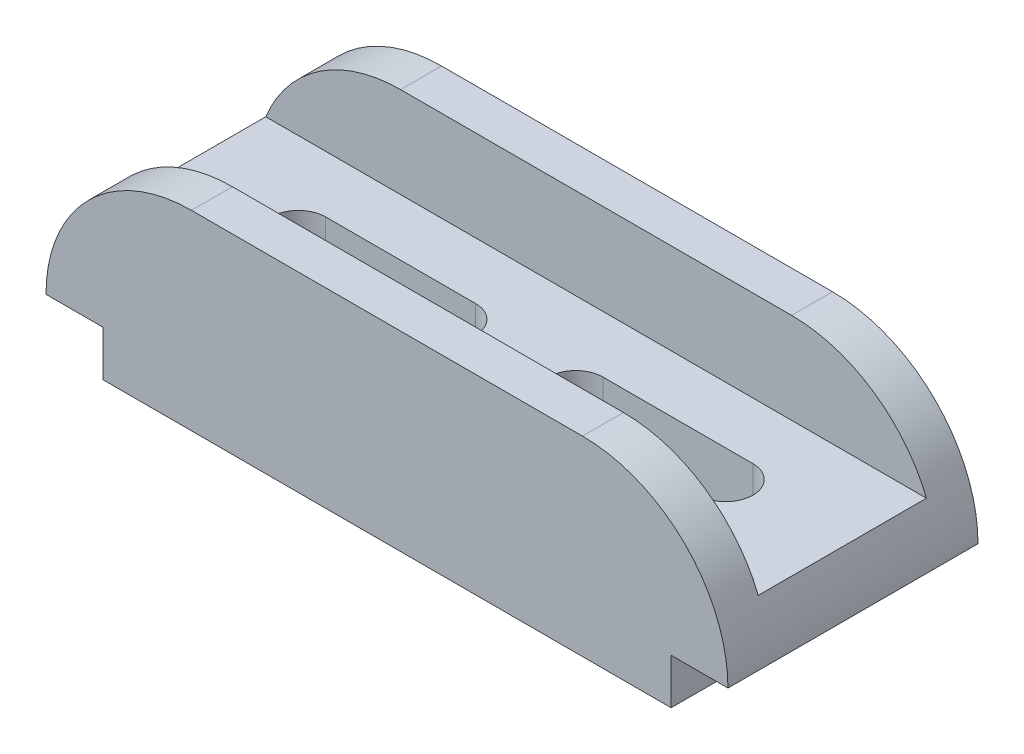
ISO-10303-21;
HEADER;
FILE_DESCRIPTION(('STEP AP214'),'2;1');
FILE_NAME('part.step','',(''),(''),'','','');
FILE_SCHEMA(('AUTOMOTIVE_DESIGN { 1 0 10303 214 1 1 1 1 }'));
ENDSEC;
DATA;
#1=APPLICATION_CONTEXT('core data for automotive mechanical design processes');
#2=APPLICATION_PROTOCOL_DEFINITION('international standard','automotive_design',2000,#1);
#3=PRODUCT_CONTEXT('',#1,'mechanical');
#4=PRODUCT('Part','Part','',(#3));
#5=PRODUCT_RELATED_PRODUCT_CATEGORY('part','',(#4));
#6=PRODUCT_DEFINITION_FORMATION('','',#4);
#7=PRODUCT_DEFINITION_CONTEXT('part definition',#1,'design');
#8=PRODUCT_DEFINITION('design','',#6,#7);
#9=PRODUCT_DEFINITION_SHAPE('','',#8);
#10=(LENGTH_UNIT() NAMED_UNIT(*) SI_UNIT(.MILLI.,.METRE.));
#11=(NAMED_UNIT(*) PLANE_ANGLE_UNIT() SI_UNIT($,.RADIAN.));
#12=(NAMED_UNIT(*) SI_UNIT($,.STERADIAN.) SOLID_ANGLE_UNIT());
#13=UNCERTAINTY_MEASURE_WITH_UNIT(LENGTH_MEASURE(1.E-05),#10,'distance_accuracy_value','');
#14=(GEOMETRIC_REPRESENTATION_CONTEXT(3) GLOBAL_UNCERTAINTY_ASSIGNED_CONTEXT((#13)) GLOBAL_UNIT_ASSIGNED_CONTEXT((#10,
#11,#12)) REPRESENTATION_CONTEXT('',''));
#15=CARTESIAN_POINT('',(0.,0.,0.));
#16=DIRECTION('',(0.,0.,1.));
#17=DIRECTION('',(1.,0.,0.));
#18=AXIS2_PLACEMENT_3D('',#15,#16,#17);
#19=CARTESIAN_POINT('',(0.,42.,27.5));
#20=DIRECTION('',(0.,-1.,0.));
#21=DIRECTION('',(1.,0.,0.));
#22=AXIS2_PLACEMENT_3D('',#19,#20,#21);
#23=PLANE('',#22);
#24=DIRECTION('',(0.,0.,-1.));
#25=VECTOR('',#24,1.);
#26=CARTESIAN_POINT('',(-43.,42.,27.5));
#27=LINE('',#26,#25);
#28=CARTESIAN_POINT('',(-43.,42.,-18.5));
#29=VERTEX_POINT('',#28);
#30=CARTESIAN_POINT('',(-43.,42.,-27.5));
#31=VERTEX_POINT('',#30);
#32=EDGE_CURVE('E314',#29,#31,#27,.T.);
#33=ORIENTED_EDGE('',*,*,#32,.F.);
#34=DIRECTION('',(-1.,0.,0.));
#35=VECTOR('',#34,1.);
#36=CARTESIAN_POINT('',(0.,42.,-18.5));
#37=LINE('',#36,#35);
#38=CARTESIAN_POINT('',(43.,42.,-18.5));
#39=VERTEX_POINT('',#38);
#40=EDGE_CURVE('E258',#39,#29,#37,.T.);
#41=ORIENTED_EDGE('',*,*,#40,.F.);
#42=DIRECTION('',(0.,0.,-1.));
#43=VECTOR('',#42,1.);
#44=CARTESIAN_POINT('',(43.,42.,27.5));
#45=LINE('',#44,#43);
#46=CARTESIAN_POINT('',(43.,42.,-27.5));
#47=VERTEX_POINT('',#46);
#48=EDGE_CURVE('E318',#39,#47,#45,.T.);
#49=ORIENTED_EDGE('',*,*,#48,.T.);
#50=DIRECTION('',(-1.,0.,0.));
#51=VECTOR('',#50,1.);
#52=CARTESIAN_POINT('',(0.,42.,-27.5));
#53=LINE('',#52,#51);
#54=EDGE_CURVE('E296',#47,#31,#53,.T.);
#55=ORIENTED_EDGE('',*,*,#54,.T.);
#56=EDGE_LOOP('',(#33,#41,#49,#55));
#57=FACE_BOUND('',#56,.T.);
#58=ADVANCED_FACE('F44',(#57),#23,.F.);
#59=CARTESIAN_POINT('',(0.,0.,27.5));
#60=DIRECTION('',(0.,1.,0.));
#61=DIRECTION('',(0.,0.,1.));
#62=AXIS2_PLACEMENT_3D('',#59,#60,#61);
#63=PLANE('',#62);
#64=DIRECTION('',(-1.,0.,0.));
#65=VECTOR('',#64,1.);
#66=CARTESIAN_POINT('',(0.,0.,-6.));
#67=LINE('',#66,#65);
#68=CARTESIAN_POINT('',(47.,0.,-6.));
#69=VERTEX_POINT('',#68);
#70=CARTESIAN_POINT('',(14.,0.,-6.));
#71=VERTEX_POINT('',#70);
#72=EDGE_CURVE('E246',#69,#71,#67,.T.);
#73=ORIENTED_EDGE('',*,*,#72,.T.);
#74=CARTESIAN_POINT('',(14.,0.,0.));
#75=DIRECTION('',(0.,1.,0.));
#76=DIRECTION('',(0.,0.,1.));
#77=AXIS2_PLACEMENT_3D('',#74,#75,#76);
#78=CIRCLE('',#77,6.);
#79=CARTESIAN_POINT('',(14.,0.,6.));
#80=VERTEX_POINT('',#79);
#81=EDGE_CURVE('E247',#71,#80,#78,.T.);
#82=ORIENTED_EDGE('',*,*,#81,.T.);
#83=DIRECTION('',(1.,0.,0.));
#84=VECTOR('',#83,1.);
#85=CARTESIAN_POINT('',(0.,0.,6.));
#86=LINE('',#85,#84);
#87=CARTESIAN_POINT('',(47.,0.,6.));
#88=VERTEX_POINT('',#87);
#89=EDGE_CURVE('E245',#80,#88,#86,.T.);
#90=ORIENTED_EDGE('',*,*,#89,.T.);
#91=CARTESIAN_POINT('',(47.,0.,0.));
#92=DIRECTION('',(0.,1.,0.));
#93=DIRECTION('',(0.,0.,1.));
#94=AXIS2_PLACEMENT_3D('',#91,#92,#93);
#95=CIRCLE('',#94,6.);
#96=EDGE_CURVE('E186',#88,#69,#95,.T.);
#97=ORIENTED_EDGE('',*,*,#96,.T.);
#98=EDGE_LOOP('',(#73,#82,#90,#97));
#99=FACE_BOUND('',#98,.T.);
#100=DIRECTION('',(-1.,0.,0.));
#101=VECTOR('',#100,1.);
#102=CARTESIAN_POINT('',(0.,0.,-5.99999999999999));
#103=LINE('',#102,#101);
#104=CARTESIAN_POINT('',(-14.,0.,-5.99999999999999));
#105=VERTEX_POINT('',#104);
#106=CARTESIAN_POINT('',(-47.,0.,-6.));
#107=VERTEX_POINT('',#106);
#108=EDGE_CURVE('E240',#105,#107,#103,.T.);
#109=ORIENTED_EDGE('',*,*,#108,.T.);
#110=CARTESIAN_POINT('',(-47.,0.,0.));
#111=DIRECTION('',(0.,1.,0.));
#112=DIRECTION('',(0.,0.,1.));
#113=AXIS2_PLACEMENT_3D('',#110,#111,#112);
#114=CIRCLE('',#113,6.);
#115=CARTESIAN_POINT('',(-47.,0.,6.));
#116=VERTEX_POINT('',#115);
#117=EDGE_CURVE('E238',#107,#116,#114,.T.);
#118=ORIENTED_EDGE('',*,*,#117,.T.);
#119=DIRECTION('',(1.,0.,0.));
#120=VECTOR('',#119,1.);
#121=CARTESIAN_POINT('',(0.,0.,5.99999999999999));
#122=LINE('',#121,#120);
#123=CARTESIAN_POINT('',(-14.,0.,6.));
#124=VERTEX_POINT('',#123);
#125=EDGE_CURVE('E211',#116,#124,#122,.T.);
#126=ORIENTED_EDGE('',*,*,#125,.T.);
#127=CARTESIAN_POINT('',(-14.,0.,0.));
#128=DIRECTION('',(0.,1.,0.));
#129=DIRECTION('',(0.,0.,1.));
#130=AXIS2_PLACEMENT_3D('',#127,#128,#129);
#131=CIRCLE('',#130,5.99999999999999);
#132=EDGE_CURVE('E232',#124,#105,#131,.T.);
#133=ORIENTED_EDGE('',*,*,#132,.T.);
#134=EDGE_LOOP('',(#109,#118,#126,#133));
#135=FACE_BOUND('',#134,.T.);
#136=DIRECTION('',(1.,0.,0.));
#137=VECTOR('',#136,1.);
#138=CARTESIAN_POINT('',(0.,0.,-27.5));
#139=LINE('',#138,#137);
#140=CARTESIAN_POINT('',(-62.5,0.,-27.5));
#141=VERTEX_POINT('',#140);
#142=CARTESIAN_POINT('',(62.5,0.,-27.5));
#143=VERTEX_POINT('',#142);
#144=EDGE_CURVE('E269',#141,#143,#139,.T.);
#145=ORIENTED_EDGE('',*,*,#144,.T.);
#146=DIRECTION('',(0.,0.,-1.));
#147=VECTOR('',#146,1.);
#148=CARTESIAN_POINT('',(62.5,0.,27.5));
#149=LINE('',#148,#147);
#150=CARTESIAN_POINT('',(62.5,0.,27.5));
#151=VERTEX_POINT('',#150);
#152=EDGE_CURVE('E327',#151,#143,#149,.T.);
#153=ORIENTED_EDGE('',*,*,#152,.F.);
#154=DIRECTION('',(1.,0.,0.));
#155=VECTOR('',#154,1.);
#156=CARTESIAN_POINT('',(0.,0.,27.5));
#157=LINE('',#156,#155);
#158=CARTESIAN_POINT('',(-62.5,0.,27.5));
#159=VERTEX_POINT('',#158);
#160=EDGE_CURVE('E271',#159,#151,#157,.T.);
#161=ORIENTED_EDGE('',*,*,#160,.F.);
#162=DIRECTION('',(0.,0.,-1.));
#163=VECTOR('',#162,1.);
#164=CARTESIAN_POINT('',(-62.5,0.,27.5));
#165=LINE('',#164,#163);
#166=EDGE_CURVE('E288',#159,#141,#165,.T.);
#167=ORIENTED_EDGE('',*,*,#166,.T.);
#168=EDGE_LOOP('',(#145,#153,#161,#167));
#169=FACE_BOUND('',#168,.T.);
#170=ADVANCED_FACE('F50',(#99,#135,#169),#63,.F.);
#171=CARTESIAN_POINT('',(62.5,0.,27.5));
#172=DIRECTION('',(-1.,0.,0.));
#173=DIRECTION('',(0.,0.,1.));
#174=AXIS2_PLACEMENT_3D('',#171,#172,#173);
#175=PLANE('',#174);
#176=DIRECTION('',(0.,1.,0.));
#177=VECTOR('',#176,1.);
#178=CARTESIAN_POINT('',(62.5,0.,-27.5));
#179=LINE('',#178,#177);
#180=CARTESIAN_POINT('',(62.5,10.,-27.5));
#181=VERTEX_POINT('',#180);
#182=EDGE_CURVE('E289',#143,#181,#179,.T.);
#183=ORIENTED_EDGE('',*,*,#182,.T.);
#184=DIRECTION('',(0.,0.,-1.));
#185=VECTOR('',#184,1.);
#186=CARTESIAN_POINT('',(62.5,10.,27.5));
#187=LINE('',#186,#185);
#188=CARTESIAN_POINT('',(62.5,10.,27.5));
#189=VERTEX_POINT('',#188);
#190=EDGE_CURVE('E324',#189,#181,#187,.T.);
#191=ORIENTED_EDGE('',*,*,#190,.F.);
#192=DIRECTION('',(0.,1.,0.));
#193=VECTOR('',#192,1.);
#194=CARTESIAN_POINT('',(62.5,0.,27.5));
#195=LINE('',#194,#193);
#196=EDGE_CURVE('E272',#151,#189,#195,.T.);
#197=ORIENTED_EDGE('',*,*,#196,.F.);
#198=ORIENTED_EDGE('',*,*,#152,.T.);
#199=EDGE_LOOP('',(#183,#191,#197,#198));
#200=FACE_BOUND('',#199,.T.);
#201=ADVANCED_FACE('F382',(#200),#175,.F.);
#202=CARTESIAN_POINT('',(62.5,10.,27.5));
#203=DIRECTION('',(0.,1.,0.));
#204=DIRECTION('',(0.,0.,1.));
#205=AXIS2_PLACEMENT_3D('',#202,#203,#204);
#206=PLANE('',#205);
#207=DIRECTION('',(1.,0.,0.));
#208=VECTOR('',#207,1.);
#209=CARTESIAN_POINT('',(62.5,10.,-27.5));
#210=LINE('',#209,#208);
#211=CARTESIAN_POINT('',(75.,10.,-27.5));
#212=VERTEX_POINT('',#211);
#213=EDGE_CURVE('E295',#181,#212,#210,.T.);
#214=ORIENTED_EDGE('',*,*,#213,.T.);
#215=DIRECTION('',(0.,0.,-1.));
#216=VECTOR('',#215,1.);
#217=CARTESIAN_POINT('',(75.,10.,27.5));
#218=LINE('',#217,#216);
#219=CARTESIAN_POINT('',(75.,10.,27.5));
#220=VERTEX_POINT('',#219);
#221=EDGE_CURVE('E325',#220,#212,#218,.T.);
#222=ORIENTED_EDGE('',*,*,#221,.F.);
#223=DIRECTION('',(1.,0.,0.));
#224=VECTOR('',#223,1.);
#225=CARTESIAN_POINT('',(62.5,10.,27.5));
#226=LINE('',#225,#224);
#227=EDGE_CURVE('E277',#189,#220,#226,.T.);
#228=ORIENTED_EDGE('',*,*,#227,.F.);
#229=ORIENTED_EDGE('',*,*,#190,.T.);
#230=EDGE_LOOP('',(#214,#222,#228,#229));
#231=FACE_BOUND('',#230,.T.);
#232=ADVANCED_FACE('F377',(#231),#206,.F.);
#233=CARTESIAN_POINT('',(43.,10.,27.5));
#234=DIRECTION('',(0.,0.,-1.));
#235=DIRECTION('',(-1.,0.,0.));
#236=AXIS2_PLACEMENT_3D('',#233,#234,#235);
#237=CYLINDRICAL_SURFACE('',#236,32.);
#238=ORIENTED_EDGE('',*,*,#48,.F.);
#239=CARTESIAN_POINT('',(43.,10.,-18.5));
#240=DIRECTION('',(0.,0.,-1.));
#241=DIRECTION('',(-1.,0.,0.));
#242=AXIS2_PLACEMENT_3D('',#239,#240,#241);
#243=CIRCLE('',#242,32.);
#244=CARTESIAN_POINT('',(72.6647939483826,22.,-18.5));
#245=VERTEX_POINT('',#244);
#246=EDGE_CURVE('E270',#39,#245,#243,.T.);
#247=ORIENTED_EDGE('',*,*,#246,.T.);
#248=DIRECTION('',(0.,0.,-1.));
#249=VECTOR('',#248,1.);
#250=CARTESIAN_POINT('',(72.6647939483827,22.,27.5));
#251=LINE('',#250,#249);
#252=CARTESIAN_POINT('',(72.6647939483827,22.,18.5));
#253=VERTEX_POINT('',#252);
#254=EDGE_CURVE('E259',#245,#253,#251,.F.);
#255=ORIENTED_EDGE('',*,*,#254,.T.);
#256=CARTESIAN_POINT('',(43.,10.,18.5));
#257=DIRECTION('',(0.,0.,1.));
#258=DIRECTION('',(1.,0.,0.));
#259=AXIS2_PLACEMENT_3D('',#256,#257,#258);
#260=CIRCLE('',#259,32.);
#261=CARTESIAN_POINT('',(43.,42.,18.5));
#262=VERTEX_POINT('',#261);
#263=EDGE_CURVE('E262',#253,#262,#260,.T.);
#264=ORIENTED_EDGE('',*,*,#263,.T.);
#265=CARTESIAN_POINT('',(43.,42.,27.5));
#266=VERTEX_POINT('',#265);
#267=EDGE_CURVE('E317',#266,#262,#45,.T.);
#268=ORIENTED_EDGE('',*,*,#267,.F.);
#269=CARTESIAN_POINT('',(43.,10.,27.5));
#270=DIRECTION('',(0.,0.,1.));
#271=DIRECTION('',(1.,0.,0.));
#272=AXIS2_PLACEMENT_3D('',#269,#270,#271);
#273=CIRCLE('',#272,32.);
#274=EDGE_CURVE('E279',#220,#266,#273,.T.);
#275=ORIENTED_EDGE('',*,*,#274,.F.);
#276=ORIENTED_EDGE('',*,*,#221,.T.);
#277=CARTESIAN_POINT('',(43.,10.,-27.5));
#278=DIRECTION('',(0.,0.,1.));
#279=DIRECTION('',(1.,0.,0.));
#280=AXIS2_PLACEMENT_3D('',#277,#278,#279);
#281=CIRCLE('',#280,32.);
#282=EDGE_CURVE('E294',#212,#47,#281,.T.);
#283=ORIENTED_EDGE('',*,*,#282,.T.);
#284=EDGE_LOOP('',(#238,#247,#255,#264,#268,#275,#276,#283));
#285=FACE_BOUND('',#284,.T.);
#286=ADVANCED_FACE('F349',(#285),#237,.T.);
#287=ORIENTED_EDGE('',*,*,#267,.T.);
#288=DIRECTION('',(1.,0.,0.));
#289=VECTOR('',#288,1.);
#290=CARTESIAN_POINT('',(92.6234355397218,42.,18.5));
#291=LINE('',#290,#289);
#292=CARTESIAN_POINT('',(-43.,42.,18.5));
#293=VERTEX_POINT('',#292);
#294=EDGE_CURVE('E252',#293,#262,#291,.T.);
#295=ORIENTED_EDGE('',*,*,#294,.F.);
#296=CARTESIAN_POINT('',(-43.,42.,27.5));
#297=VERTEX_POINT('',#296);
#298=EDGE_CURVE('E312',#297,#293,#27,.T.);
#299=ORIENTED_EDGE('',*,*,#298,.F.);
#300=DIRECTION('',(-1.,0.,0.));
#301=VECTOR('',#300,1.);
#302=CARTESIAN_POINT('',(0.,42.,27.5));
#303=LINE('',#302,#301);
#304=EDGE_CURVE('E278',#266,#297,#303,.T.);
#305=ORIENTED_EDGE('',*,*,#304,.F.);
#306=EDGE_LOOP('',(#287,#295,#299,#305));
#307=FACE_BOUND('',#306,.T.);
#308=ADVANCED_FACE('F343',(#307),#23,.F.);
#309=CARTESIAN_POINT('',(-43.,10.,27.5));
#310=DIRECTION('',(0.,0.,-1.));
#311=DIRECTION('',(-1.,0.,0.));
#312=AXIS2_PLACEMENT_3D('',#309,#310,#311);
#313=CYLINDRICAL_SURFACE('',#312,32.);
#314=DIRECTION('',(0.,0.,-1.));
#315=VECTOR('',#314,1.);
#316=CARTESIAN_POINT('',(-72.6647939483826,22.,27.5));
#317=LINE('',#316,#315);
#318=CARTESIAN_POINT('',(-72.6647939483826,22.,18.5));
#319=VERTEX_POINT('',#318);
#320=CARTESIAN_POINT('',(-72.6647939483826,22.,-18.5));
#321=VERTEX_POINT('',#320);
#322=EDGE_CURVE('E332',#319,#321,#317,.T.);
#323=ORIENTED_EDGE('',*,*,#322,.T.);
#324=CARTESIAN_POINT('',(-43.,10.,-18.5));
#325=DIRECTION('',(0.,0.,-1.));
#326=DIRECTION('',(-1.,0.,0.));
#327=AXIS2_PLACEMENT_3D('',#324,#325,#326);
#328=CIRCLE('',#327,32.);
#329=EDGE_CURVE('E11',#321,#29,#328,.T.);
#330=ORIENTED_EDGE('',*,*,#329,.T.);
#331=ORIENTED_EDGE('',*,*,#32,.T.);
#332=CARTESIAN_POINT('',(-43.,10.,-27.5));
#333=DIRECTION('',(0.,0.,1.));
#334=DIRECTION('',(1.,0.,0.));
#335=AXIS2_PLACEMENT_3D('',#332,#333,#334);
#336=CIRCLE('',#335,32.);
#337=CARTESIAN_POINT('',(-75.,10.,-27.5));
#338=VERTEX_POINT('',#337);
#339=EDGE_CURVE('E297',#31,#338,#336,.T.);
#340=ORIENTED_EDGE('',*,*,#339,.T.);
#341=DIRECTION('',(0.,0.,-1.));
#342=VECTOR('',#341,1.);
#343=CARTESIAN_POINT('',(-75.,10.,27.5));
#344=LINE('',#343,#342);
#345=CARTESIAN_POINT('',(-75.,10.,27.5));
#346=VERTEX_POINT('',#345);
#347=EDGE_CURVE('E313',#346,#338,#344,.T.);
#348=ORIENTED_EDGE('',*,*,#347,.F.);
#349=CARTESIAN_POINT('',(-43.,10.,27.5));
#350=DIRECTION('',(0.,0.,1.));
#351=DIRECTION('',(1.,0.,0.));
#352=AXIS2_PLACEMENT_3D('',#349,#350,#351);
#353=CIRCLE('',#352,32.);
#354=EDGE_CURVE('E281',#297,#346,#353,.T.);
#355=ORIENTED_EDGE('',*,*,#354,.F.);
#356=ORIENTED_EDGE('',*,*,#298,.T.);
#357=CARTESIAN_POINT('',(-43.,10.,18.5));
#358=DIRECTION('',(0.,0.,1.));
#359=DIRECTION('',(1.,0.,0.));
#360=AXIS2_PLACEMENT_3D('',#357,#358,#359);
#361=CIRCLE('',#360,32.);
#362=EDGE_CURVE('E52',#293,#319,#361,.T.);
#363=ORIENTED_EDGE('',*,*,#362,.T.);
#364=EDGE_LOOP('',(#323,#330,#331,#340,#348,#355,#356,#363));
#365=FACE_BOUND('',#364,.T.);
#366=ADVANCED_FACE('F333',(#365),#313,.T.);
#367=CARTESIAN_POINT('',(-62.5,10.,27.5));
#368=DIRECTION('',(0.,1.,0.));
#369=DIRECTION('',(0.,0.,1.));
#370=AXIS2_PLACEMENT_3D('',#367,#368,#369);
#371=PLANE('',#370);
#372=DIRECTION('',(1.,0.,0.));
#373=VECTOR('',#372,1.);
#374=CARTESIAN_POINT('',(-62.5,10.,-27.5));
#375=LINE('',#374,#373);
#376=CARTESIAN_POINT('',(-62.5,10.,-27.5));
#377=VERTEX_POINT('',#376);
#378=EDGE_CURVE('E305',#338,#377,#375,.T.);
#379=ORIENTED_EDGE('',*,*,#378,.T.);
#380=DIRECTION('',(0.,0.,-1.));
#381=VECTOR('',#380,1.);
#382=CARTESIAN_POINT('',(-62.5,10.,27.5));
#383=LINE('',#382,#381);
#384=CARTESIAN_POINT('',(-62.5,10.,27.5));
#385=VERTEX_POINT('',#384);
#386=EDGE_CURVE('E306',#385,#377,#383,.T.);
#387=ORIENTED_EDGE('',*,*,#386,.F.);
#388=DIRECTION('',(1.,0.,0.));
#389=VECTOR('',#388,1.);
#390=CARTESIAN_POINT('',(-62.5,10.,27.5));
#391=LINE('',#390,#389);
#392=EDGE_CURVE('E283',#346,#385,#391,.T.);
#393=ORIENTED_EDGE('',*,*,#392,.F.);
#394=ORIENTED_EDGE('',*,*,#347,.T.);
#395=EDGE_LOOP('',(#379,#387,#393,#394));
#396=FACE_BOUND('',#395,.T.);
#397=ADVANCED_FACE('F366',(#396),#371,.F.);
#398=CARTESIAN_POINT('',(-62.5,0.,27.5));
#399=DIRECTION('',(1.,0.,0.));
#400=DIRECTION('',(0.,0.,-1.));
#401=AXIS2_PLACEMENT_3D('',#398,#399,#400);
#402=PLANE('',#401);
#403=DIRECTION('',(0.,-1.,0.));
#404=VECTOR('',#403,1.);
#405=CARTESIAN_POINT('',(-62.5,0.,-27.5));
#406=LINE('',#405,#404);
#407=EDGE_CURVE('E273',#377,#141,#406,.T.);
#408=ORIENTED_EDGE('',*,*,#407,.T.);
#409=ORIENTED_EDGE('',*,*,#166,.F.);
#410=DIRECTION('',(0.,-1.,0.));
#411=VECTOR('',#410,1.);
#412=CARTESIAN_POINT('',(-62.5,0.,27.5));
#413=LINE('',#412,#411);
#414=EDGE_CURVE('E286',#385,#159,#413,.T.);
#415=ORIENTED_EDGE('',*,*,#414,.F.);
#416=ORIENTED_EDGE('',*,*,#386,.T.);
#417=EDGE_LOOP('',(#408,#409,#415,#416));
#418=FACE_BOUND('',#417,.T.);
#419=ADVANCED_FACE('F389',(#418),#402,.F.);
#420=CARTESIAN_POINT('',(-43.,10.,27.5));
#421=DIRECTION('',(0.,0.,1.));
#422=DIRECTION('',(1.,0.,0.));
#423=AXIS2_PLACEMENT_3D('',#420,#421,#422);
#424=PLANE('',#423);
#425=ORIENTED_EDGE('',*,*,#160,.T.);
#426=ORIENTED_EDGE('',*,*,#196,.T.);
#427=ORIENTED_EDGE('',*,*,#227,.T.);
#428=ORIENTED_EDGE('',*,*,#274,.T.);
#429=ORIENTED_EDGE('',*,*,#304,.T.);
#430=ORIENTED_EDGE('',*,*,#354,.T.);
#431=ORIENTED_EDGE('',*,*,#392,.T.);
#432=ORIENTED_EDGE('',*,*,#414,.T.);
#433=EDGE_LOOP('',(#425,#426,#427,#428,#429,#430,#431,#432));
#434=FACE_BOUND('',#433,.T.);
#435=ADVANCED_FACE('F375',(#434),#424,.T.);
#436=CARTESIAN_POINT('',(-43.,10.,-27.5));
#437=DIRECTION('',(0.,0.,1.));
#438=DIRECTION('',(1.,0.,0.));
#439=AXIS2_PLACEMENT_3D('',#436,#437,#438);
#440=PLANE('',#439);
#441=ORIENTED_EDGE('',*,*,#144,.F.);
#442=ORIENTED_EDGE('',*,*,#407,.F.);
#443=ORIENTED_EDGE('',*,*,#378,.F.);
#444=ORIENTED_EDGE('',*,*,#339,.F.);
#445=ORIENTED_EDGE('',*,*,#54,.F.);
#446=ORIENTED_EDGE('',*,*,#282,.F.);
#447=ORIENTED_EDGE('',*,*,#213,.F.);
#448=ORIENTED_EDGE('',*,*,#182,.F.);
#449=EDGE_LOOP('',(#441,#442,#443,#444,#445,#446,#447,#448));
#450=FACE_BOUND('',#449,.T.);
#451=ADVANCED_FACE('F361',(#450),#440,.F.);
#452=CARTESIAN_POINT('',(0.,22.,-18.5));
#453=DIRECTION('',(0.,0.,-1.));
#454=DIRECTION('',(-1.,0.,0.));
#455=AXIS2_PLACEMENT_3D('',#452,#453,#454);
#456=PLANE('',#455);
#457=ORIENTED_EDGE('',*,*,#40,.T.);
#458=ORIENTED_EDGE('',*,*,#329,.F.);
#459=DIRECTION('',(-1.,0.,0.));
#460=VECTOR('',#459,1.);
#461=CARTESIAN_POINT('',(-101.990097212072,22.,-18.5));
#462=LINE('',#461,#460);
#463=EDGE_CURVE('E251',#245,#321,#462,.T.);
#464=ORIENTED_EDGE('',*,*,#463,.F.);
#465=ORIENTED_EDGE('',*,*,#246,.F.);
#466=EDGE_LOOP('',(#457,#458,#464,#465));
#467=FACE_BOUND('',#466,.T.);
#468=ADVANCED_FACE('F353',(#467),#456,.F.);
#469=CARTESIAN_POINT('',(92.6234355397218,22.,18.5));
#470=DIRECTION('',(0.,0.,1.));
#471=DIRECTION('',(1.,0.,0.));
#472=AXIS2_PLACEMENT_3D('',#469,#470,#471);
#473=PLANE('',#472);
#474=DIRECTION('',(1.,0.,0.));
#475=VECTOR('',#474,1.);
#476=CARTESIAN_POINT('',(92.6234355397218,22.,18.5));
#477=LINE('',#476,#475);
#478=EDGE_CURVE('E254',#319,#253,#477,.T.);
#479=ORIENTED_EDGE('',*,*,#478,.F.);
#480=ORIENTED_EDGE('',*,*,#362,.F.);
#481=ORIENTED_EDGE('',*,*,#294,.T.);
#482=ORIENTED_EDGE('',*,*,#263,.F.);
#483=EDGE_LOOP('',(#479,#480,#481,#482));
#484=FACE_BOUND('',#483,.T.);
#485=ADVANCED_FACE('F341',(#484),#473,.F.);
#486=CARTESIAN_POINT('',(0.,22.,0.));
#487=DIRECTION('',(0.,-1.,0.));
#488=DIRECTION('',(1.,0.,0.));
#489=AXIS2_PLACEMENT_3D('',#486,#487,#488);
#490=PLANE('',#489);
#491=DIRECTION('',(1.,0.,0.));
#492=VECTOR('',#491,1.);
#493=CARTESIAN_POINT('',(14.,22.,6.));
#494=LINE('',#493,#492);
#495=CARTESIAN_POINT('',(14.,22.,6.));
#496=VERTEX_POINT('',#495);
#497=CARTESIAN_POINT('',(47.,22.,6.));
#498=VERTEX_POINT('',#497);
#499=EDGE_CURVE('E192',#496,#498,#494,.T.);
#500=ORIENTED_EDGE('',*,*,#499,.F.);
#501=CARTESIAN_POINT('',(14.,22.,0.));
#502=DIRECTION('',(0.,1.,0.));
#503=DIRECTION('',(-1.,0.,0.));
#504=AXIS2_PLACEMENT_3D('',#501,#502,#503);
#505=CIRCLE('',#504,6.);
#506=CARTESIAN_POINT('',(14.,22.,-6.));
#507=VERTEX_POINT('',#506);
#508=EDGE_CURVE('E200',#507,#496,#505,.T.);
#509=ORIENTED_EDGE('',*,*,#508,.F.);
#510=DIRECTION('',(-1.,0.,0.));
#511=VECTOR('',#510,1.);
#512=CARTESIAN_POINT('',(14.,22.,-6.));
#513=LINE('',#512,#511);
#514=CARTESIAN_POINT('',(47.,22.,-6.));
#515=VERTEX_POINT('',#514);
#516=EDGE_CURVE('E204',#515,#507,#513,.T.);
#517=ORIENTED_EDGE('',*,*,#516,.F.);
#518=CARTESIAN_POINT('',(47.,22.,0.));
#519=DIRECTION('',(0.,1.,0.));
#520=DIRECTION('',(-1.,0.,0.));
#521=AXIS2_PLACEMENT_3D('',#518,#519,#520);
#522=CIRCLE('',#521,6.);
#523=EDGE_CURVE('E184',#498,#515,#522,.T.);
#524=ORIENTED_EDGE('',*,*,#523,.F.);
#525=EDGE_LOOP('',(#500,#509,#517,#524));
#526=FACE_BOUND('',#525,.T.);
#527=DIRECTION('',(1.,0.,0.));
#528=VECTOR('',#527,1.);
#529=CARTESIAN_POINT('',(-14.,22.,5.99999999999999));
#530=LINE('',#529,#528);
#531=CARTESIAN_POINT('',(-47.,22.,6.));
#532=VERTEX_POINT('',#531);
#533=CARTESIAN_POINT('',(-14.,22.,5.99999999999999));
#534=VERTEX_POINT('',#533);
#535=EDGE_CURVE('E216',#532,#534,#530,.T.);
#536=ORIENTED_EDGE('',*,*,#535,.F.);
#537=CARTESIAN_POINT('',(-47.,22.,0.));
#538=DIRECTION('',(0.,1.,0.));
#539=DIRECTION('',(1.,0.,0.));
#540=AXIS2_PLACEMENT_3D('',#537,#538,#539);
#541=CIRCLE('',#540,6.);
#542=CARTESIAN_POINT('',(-47.,22.,-6.));
#543=VERTEX_POINT('',#542);
#544=EDGE_CURVE('E212',#543,#532,#541,.T.);
#545=ORIENTED_EDGE('',*,*,#544,.F.);
#546=DIRECTION('',(-1.,0.,0.));
#547=VECTOR('',#546,1.);
#548=CARTESIAN_POINT('',(-14.,22.,-5.99999999999999));
#549=LINE('',#548,#547);
#550=CARTESIAN_POINT('',(-14.,22.,-5.99999999999999));
#551=VERTEX_POINT('',#550);
#552=EDGE_CURVE('E222',#551,#543,#549,.T.);
#553=ORIENTED_EDGE('',*,*,#552,.F.);
#554=CARTESIAN_POINT('',(-14.,22.,0.));
#555=DIRECTION('',(0.,1.,0.));
#556=DIRECTION('',(1.,0.,0.));
#557=AXIS2_PLACEMENT_3D('',#554,#555,#556);
#558=CIRCLE('',#557,5.99999999999999);
#559=EDGE_CURVE('E217',#534,#551,#558,.T.);
#560=ORIENTED_EDGE('',*,*,#559,.F.);
#561=EDGE_LOOP('',(#536,#545,#553,#560));
#562=FACE_BOUND('',#561,.T.);
#563=ORIENTED_EDGE('',*,*,#463,.T.);
#564=ORIENTED_EDGE('',*,*,#322,.F.);
#565=ORIENTED_EDGE('',*,*,#478,.T.);
#566=ORIENTED_EDGE('',*,*,#254,.F.);
#567=EDGE_LOOP('',(#563,#564,#565,#566));
#568=FACE_BOUND('',#567,.T.);
#569=ADVANCED_FACE('F203',(#526,#562,#568),#490,.F.);
#570=CARTESIAN_POINT('',(-47.,-16.,0.));
#571=DIRECTION('',(0.,1.,0.));
#572=DIRECTION('',(-1.,0.,0.));
#573=AXIS2_PLACEMENT_3D('',#570,#571,#572);
#574=CYLINDRICAL_SURFACE('',#573,6.);
#575=DIRECTION('',(0.,1.,0.));
#576=VECTOR('',#575,1.);
#577=CARTESIAN_POINT('',(-47.,-16.,-6.));
#578=LINE('',#577,#576);
#579=EDGE_CURVE('E223',#107,#543,#578,.T.);
#580=ORIENTED_EDGE('',*,*,#579,.T.);
#581=ORIENTED_EDGE('',*,*,#544,.T.);
#582=DIRECTION('',(0.,1.,0.));
#583=VECTOR('',#582,1.);
#584=CARTESIAN_POINT('',(-47.,-16.,6.));
#585=LINE('',#584,#583);
#586=EDGE_CURVE('E221',#116,#532,#585,.T.);
#587=ORIENTED_EDGE('',*,*,#586,.F.);
#588=ORIENTED_EDGE('',*,*,#117,.F.);
#589=EDGE_LOOP('',(#580,#581,#587,#588));
#590=FACE_BOUND('',#589,.T.);
#591=ADVANCED_FACE('F486',(#590),#574,.F.);
#592=CARTESIAN_POINT('',(-14.,-16.,-5.99999999999999));
#593=DIRECTION('',(0.,0.,-1.));
#594=DIRECTION('',(-1.,0.,0.));
#595=AXIS2_PLACEMENT_3D('',#592,#593,#594);
#596=PLANE('',#595);
#597=DIRECTION('',(0.,1.,0.));
#598=VECTOR('',#597,1.);
#599=CARTESIAN_POINT('',(-14.,-16.,-5.99999999999999));
#600=LINE('',#599,#598);
#601=EDGE_CURVE('E226',#105,#551,#600,.T.);
#602=ORIENTED_EDGE('',*,*,#601,.T.);
#603=ORIENTED_EDGE('',*,*,#552,.T.);
#604=ORIENTED_EDGE('',*,*,#579,.F.);
#605=ORIENTED_EDGE('',*,*,#108,.F.);
#606=EDGE_LOOP('',(#602,#603,#604,#605));
#607=FACE_BOUND('',#606,.T.);
#608=ADVANCED_FACE('F497',(#607),#596,.F.);
#609=CARTESIAN_POINT('',(-14.,-16.,0.));
#610=DIRECTION('',(0.,1.,0.));
#611=DIRECTION('',(-1.,0.,0.));
#612=AXIS2_PLACEMENT_3D('',#609,#610,#611);
#613=CYLINDRICAL_SURFACE('',#612,5.99999999999999);
#614=DIRECTION('',(0.,1.,0.));
#615=VECTOR('',#614,1.);
#616=CARTESIAN_POINT('',(-14.,-16.,5.99999999999999));
#617=LINE('',#616,#615);
#618=EDGE_CURVE('E68',#124,#534,#617,.T.);
#619=ORIENTED_EDGE('',*,*,#618,.T.);
#620=ORIENTED_EDGE('',*,*,#559,.T.);
#621=ORIENTED_EDGE('',*,*,#601,.F.);
#622=ORIENTED_EDGE('',*,*,#132,.F.);
#623=EDGE_LOOP('',(#619,#620,#621,#622));
#624=FACE_BOUND('',#623,.T.);
#625=ADVANCED_FACE('F508',(#624),#613,.F.);
#626=CARTESIAN_POINT('',(-14.,-16.,5.99999999999999));
#627=DIRECTION('',(0.,0.,1.));
#628=DIRECTION('',(1.,0.,0.));
#629=AXIS2_PLACEMENT_3D('',#626,#627,#628);
#630=PLANE('',#629);
#631=ORIENTED_EDGE('',*,*,#586,.T.);
#632=ORIENTED_EDGE('',*,*,#535,.T.);
#633=ORIENTED_EDGE('',*,*,#618,.F.);
#634=ORIENTED_EDGE('',*,*,#125,.F.);
#635=EDGE_LOOP('',(#631,#632,#633,#634));
#636=FACE_BOUND('',#635,.T.);
#637=ADVANCED_FACE('F517',(#636),#630,.F.);
#638=CARTESIAN_POINT('',(14.,-16.,0.));
#639=DIRECTION('',(0.,1.,0.));
#640=DIRECTION('',(-1.,0.,0.));
#641=AXIS2_PLACEMENT_3D('',#638,#639,#640);
#642=CYLINDRICAL_SURFACE('',#641,6.);
#643=DIRECTION('',(0.,1.,0.));
#644=VECTOR('',#643,1.);
#645=CARTESIAN_POINT('',(14.,-16.,-6.));
#646=LINE('',#645,#644);
#647=EDGE_CURVE('E207',#71,#507,#646,.T.);
#648=ORIENTED_EDGE('',*,*,#647,.T.);
#649=ORIENTED_EDGE('',*,*,#508,.T.);
#650=DIRECTION('',(0.,1.,0.));
#651=VECTOR('',#650,1.);
#652=CARTESIAN_POINT('',(14.,-16.,6.));
#653=LINE('',#652,#651);
#654=EDGE_CURVE('E187',#80,#496,#653,.T.);
#655=ORIENTED_EDGE('',*,*,#654,.F.);
#656=ORIENTED_EDGE('',*,*,#81,.F.);
#657=EDGE_LOOP('',(#648,#649,#655,#656));
#658=FACE_BOUND('',#657,.T.);
#659=ADVANCED_FACE('F535',(#658),#642,.F.);
#660=CARTESIAN_POINT('',(14.,-16.,-6.));
#661=DIRECTION('',(0.,0.,-1.));
#662=DIRECTION('',(-1.,0.,0.));
#663=AXIS2_PLACEMENT_3D('',#660,#661,#662);
#664=PLANE('',#663);
#665=DIRECTION('',(0.,1.,0.));
#666=VECTOR('',#665,1.);
#667=CARTESIAN_POINT('',(47.,-16.,-6.));
#668=LINE('',#667,#666);
#669=EDGE_CURVE('E188',#69,#515,#668,.T.);
#670=ORIENTED_EDGE('',*,*,#669,.T.);
#671=ORIENTED_EDGE('',*,*,#516,.T.);
#672=ORIENTED_EDGE('',*,*,#647,.F.);
#673=ORIENTED_EDGE('',*,*,#72,.F.);
#674=EDGE_LOOP('',(#670,#671,#672,#673));
#675=FACE_BOUND('',#674,.T.);
#676=ADVANCED_FACE('F543',(#675),#664,.F.);
#677=CARTESIAN_POINT('',(47.,-16.,0.));
#678=DIRECTION('',(0.,1.,0.));
#679=DIRECTION('',(-1.,0.,0.));
#680=AXIS2_PLACEMENT_3D('',#677,#678,#679);
#681=CYLINDRICAL_SURFACE('',#680,6.);
#682=DIRECTION('',(0.,1.,0.));
#683=VECTOR('',#682,1.);
#684=CARTESIAN_POINT('',(47.,-16.,6.));
#685=LINE('',#684,#683);
#686=EDGE_CURVE('E58',#88,#498,#685,.T.);
#687=ORIENTED_EDGE('',*,*,#686,.T.);
#688=ORIENTED_EDGE('',*,*,#523,.T.);
#689=ORIENTED_EDGE('',*,*,#669,.F.);
#690=ORIENTED_EDGE('',*,*,#96,.F.);
#691=EDGE_LOOP('',(#687,#688,#689,#690));
#692=FACE_BOUND('',#691,.T.);
#693=ADVANCED_FACE('F182',(#692),#681,.F.);
#694=CARTESIAN_POINT('',(14.,-16.,6.));
#695=DIRECTION('',(0.,0.,1.));
#696=DIRECTION('',(1.,0.,0.));
#697=AXIS2_PLACEMENT_3D('',#694,#695,#696);
#698=PLANE('',#697);
#699=ORIENTED_EDGE('',*,*,#654,.T.);
#700=ORIENTED_EDGE('',*,*,#499,.T.);
#701=ORIENTED_EDGE('',*,*,#686,.F.);
#702=ORIENTED_EDGE('',*,*,#89,.F.);
#703=EDGE_LOOP('',(#699,#700,#701,#702));
#704=FACE_BOUND('',#703,.T.);
#705=ADVANCED_FACE('F194',(#704),#698,.F.);
#706=CLOSED_SHELL('',(#58,#170,#201,#232,#286,#308,#366,#397,#419,#435,#451,#468,#485,#569,#591,
#608,#625,#637,#659,#676,#693,#705));
#707=MANIFOLD_SOLID_BREP('B2',#706);
#708=ADVANCED_BREP_SHAPE_REPRESENTATION('',(#18,#707),#14);
#709=SHAPE_DEFINITION_REPRESENTATION(#9,#708);
ENDSEC;
END-ISO-10303-21;
